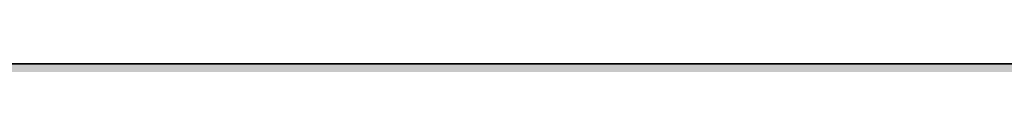
# Model space of a CAD drawing. Units: inches. Extents: x 2091 to 2899, y 967 to 2217.
# Tile 102 of 256: x 2252.951 to 2253.5204, y 1099.9191 to 1099.9191. Entities that reach past the tile are written whole.
import ezdxf

# ---------------------------------------------------------------- set-up
doc = ezdxf.new("R2010")
doc.units = ezdxf.units.IN
doc.layers.add('A-WALL-PATT', color=141, linetype='Continuous', lineweight=13, true_color=0xadddf7)
doc.layers.add('L-SITE-WALL', color=7, linetype='Continuous', lineweight=35)

msp = doc.modelspace()

# ---------------------------------------------------------------- hatches: boundary and pattern name
at = {"layer": 'A-WALL-PATT'}
h = msp.add_hatch(color=256, dxfattribs=at)
h.dxf.hatch_style = 1
h.paths.add_polyline_path([(2212.1436, 1941.41906), (2387.6436, 1941.41906), (2387.6436, 1824.41906), (2392.1436, 1824.41906), (2392.1436, 1941.41906), (2609.6436, 1941.41906), (2609.6436, 1825.91906), (2614.1436, 1825.91906), (2614.1436, 1941.41906), (2794.1436, 1941.41906), (2794.1436, 1928.76217), (2803.1436, 1928.76217), (2803.1436, 2050.91906), (2203.1436, 2050.91906), (2203.1436, 1900.75786), (2212.1436, 1900.75786)])
h.paths.add_polyline_path([(2212.1436, 1945.91906), (2212.1436, 2041.91906), (2794.1436, 2041.91906), (2794.1436, 1945.91906), (2402.24824, 1945.91906), (2401.10243, 1945.77583), (2398.70243, 1945.77583)], flags=16)
h.paths.add_polyline_path([(2230.22986, 1948.06279), (2227.34986, 1949.50279), (2225.90986, 1951.90279), (2223.98986, 1952.86279), (2223.02986, 1955.26279), (2222.06986, 1959.58279), (2222.06986, 1963.42279), (2223.02986, 1965.66279), (2223.98986, 1965.34279), (2225.58591, 1963.86075), (2226.91153, 1964.95726), (2226.94886, 1965.93879), (2227.77832, 1966.95214), (2228.19992, 1968.8787), (2230.70986, 1964.86279), (2233.58986, 1966.30279), (2233.60731, 1966.33187), (2233.77266, 1964.9382), (2234.6338, 1963.67647), (2235.02986, 1963.90279), (2236.28203, 1965.57236), (2235.98986, 1962.94279), (2237.95451, 1957.54), (2238.38986, 1957.90279), (2239.21586, 1960.30579), (2238.65457, 1966.38496), (2238.69279, 1966.43807), (2238.84058, 1967.49971), (2238.78029, 1967.68749), (2238.88054, 1967.78676), (2238.66686, 1966.25179), (2239.21586, 1960.30579), (2238.38986, 1957.90279), (2236.94986, 1956.70279), (2234.54986, 1949.98279)], flags=0)
h.paths.add_polyline_path([(2278.01197, 1948.06279), (2276.49643, 1947.87335), (2275.84983, 1947.68861), (2274.65197, 1947.10279)], flags=0)
h.paths.add_polyline_path([(2269.85197, 1955.74279), (2268.27618, 1956.62933), (2270.8673, 1956.3484), (2269.37197, 1958.14279), (2268.71496, 1959.19233), (2270.56983, 1958.72861), (2268.58073, 1961.90609), (2270.81197, 1960.89188), (2270.81197, 1963.42279), (2271.39331, 1964.77926), (2270.29176, 1966.1562), (2271.77197, 1965.66279), (2272.14139, 1966.52476), (2273.92983, 1965.92861), (2275.63039, 1968.0543), (2276.33194, 1966.72186), (2276.52043, 1966.95214), (2276.94203, 1968.8787), (2277.73429, 1967.61108), (2278.13989, 1969.46452), (2279.65912, 1967.03374), (2280.41197, 1966.78279), (2280.9493, 1967.58879), (2281.60983, 1967.36861), (2282.13327, 1968.15376), (2282.34924, 1966.33344), (2282.34985, 1966.33259), (2283.40755, 1968.09542), (2283.71263, 1965.52402), (2284.32022, 1964.63379), (2284.51181, 1964.88924), (2284.23497, 1965.70479), (2284.50047, 1967.31896), (2284.90794, 1965.41742), (2285.39631, 1966.06858), (2285.43283, 1966.29061), (2285.47334, 1966.17128), (2286.35392, 1967.34539), (2286.22201, 1966.15817), (2287.66349, 1968.08015), (2287.71397, 1968.44279), (2288.4816, 1969.01668), (2288.57399, 1968.7289), (2288.91746, 1969.06904), (2288.60683, 1966.83761), (2288.92873, 1963.35131), (2288.93497, 1963.35679), (2288.92973, 1963.34042), (2289.01528, 1962.41387), (2290.11122, 1963.87513), (2290.13283, 1963.94261), (2290.21767, 1964.01706), (2290.11122, 1963.87513), (2289.15583, 1960.89161), (2288.59404, 1959.25723), (2288.57197, 1959.10279), (2289.53197, 1960.54279), (2290.01197, 1962.46279), (2290.19184, 1962.64266), (2289.76983, 1959.68861), (2286.88983, 1957.28861), (2284.48983, 1950.56861), (2283.31466, 1950.04631), (2283.29197, 1949.98279), (2280.29006, 1948.64861), (2281.12983, 1948.64861), (2282.56983, 1948.16861), (2283.20473, 1948.06279), (2278.97197, 1948.06279), (2276.09197, 1949.50279), (2274.65197, 1951.90279), (2272.73197, 1952.86279)], flags=0)
h.paths.add_polyline_path([(2271.15887, 1958.02177), (2272.96983, 1955.84861), (2272.00983, 1960.16861), (2272.00983, 1964.00861), (2272.62443, 1965.44266), (2274.32802, 1963.86075), (2275.65365, 1964.95726), (2275.63774, 1964.53909), (2277.41223, 1966.00689), (2277.03297, 1965.15679), (2276.82992, 1964.9756), (2276.76601, 1963.29501), (2277.44964, 1962.66022), (2279.45197, 1964.86279), (2282.33197, 1966.30279), (2283.52983, 1966.88861), (2283.29451, 1966.77095), (2283.91299, 1963.8847), (2284.89925, 1964.44827), (2284.73197, 1962.94279), (2286.69662, 1957.54), (2287.13197, 1957.90279), (2287.54191, 1959.09539), (2287.7794, 1958.44231), (2285.68274, 1956.6951), (2285.8765, 1959.79534), (2284.73197, 1962.94279), (2284.89925, 1964.44827), (2283.91299, 1963.8847), (2284.22383, 1962.43412), (2283.42436, 1963.60548), (2281.60983, 1962.56861), (2281.12983, 1960.16861), (2282.08983, 1956.32861), (2283.04983, 1952.96861), (2282.56983, 1950.56861), (2280.16983, 1948.64861), (2279.88332, 1948.79187), (2278.97197, 1948.06279), (2278.97197, 1949.02279), (2278.67231, 1949.39737), (2277.28983, 1950.08861), (2275.84983, 1952.48861), (2273.92983, 1953.44861), (2272.48983, 1954.88861), (2271.92165, 1954.88861), (2271.77197, 1955.26279)], flags=0)
h.paths.add_polyline_path([(2311.99415, 1955.74279), (2312.06272, 1955.67422), (2312.0551, 1955.7085)], flags=0)
h.paths.add_polyline_path([(2331.95615, 1963.95179), (2333.39615, 1965.39179), (2331.07715, 1963.35679), (2330.9986, 1963.11152)], flags=0)
h.paths.add_polyline_path([(2310.55415, 1954.30279), (2307.03981, 1956.27994), (2310.7629, 1955.87628), (2312.47415, 1953.82279), (2313.43415, 1951.42279), (2315.35415, 1950.46279), (2316.79415, 1948.06279), (2317.46615, 1947.72679), (2319.36869, 1947.96461), (2317.75415, 1949.98279), (2317.56953, 1950.61048), (2316.79415, 1951.90279), (2314.87415, 1952.86279), (2313.91415, 1955.26279), (2311.51415, 1958.14279), (2309.37549, 1961.55917), (2311.51415, 1960.33708), (2311.51415, 1961.98279), (2310.60467, 1963.11963), (2311.72661, 1962.47853), (2312.41833, 1964.09256), (2312.25596, 1964.29552), (2313.19415, 1963.98279), (2313.91415, 1965.66279), (2314.64678, 1965.41858), (2315.35415, 1966.30279), (2316.79415, 1967.74279), (2316.15744, 1966.9469), (2317.03411, 1965.28186), (2317.2226, 1965.51214), (2317.77705, 1968.04577), (2318.47411, 1966.72186), (2318.6626, 1966.95214), (2319.0842, 1968.8787), (2321.20705, 1965.48215), (2322.16142, 1966.9137), (2322.55415, 1966.78279), (2322.78599, 1967.13056), (2322.88165, 1966.32429), (2323.31204, 1965.72174), (2323.65129, 1965.89136), (2324.3965, 1967.13338), (2324.65694, 1964.9382), (2324.97199, 1964.47661), (2325.38728, 1967.0015), (2325.94081, 1964.41835), (2327.22893, 1966.13584), (2327.16632, 1965.57236), (2328.05914, 1966.76278), (2328.22458, 1966.24749), (2329.66797, 1967.67691), (2329.66458, 1967.68749), (2329.76482, 1967.78676), (2329.55115, 1966.25179), (2330.10015, 1960.30579), (2329.33281, 1958.07347), (2329.31306, 1957.93523), (2329.63415, 1958.20279), (2330.23415, 1959.10279), (2330.71415, 1961.02279), (2331.03415, 1961.34279), (2330.71415, 1959.10279), (2329.63415, 1958.20279), (2329.27415, 1957.66279), (2327.71211, 1956.3611), (2325.43415, 1949.98279), (2324.33377, 1949.49374), (2323.99415, 1948.54279), (2319.67415, 1946.62279), (2316.79415, 1948.06279), (2315.35415, 1950.46279), (2313.43415, 1951.42279)], flags=0)
h.paths.add_polyline_path([(2321.33568, 1947.95202), (2321.11415, 1948.06279), (2321.11415, 1949.02279), (2319.19415, 1951.42279), (2316.79415, 1959.58279), (2316.66324, 1959.58279), (2315.35415, 1958.14279), (2314.39415, 1958.14279), (2313.1483, 1958.70908), (2312.95415, 1959.58279), (2312.95415, 1960.89188), (2315.83415, 1959.58279), (2316.66324, 1959.58279), (2317.31471, 1960.29941), (2315.0302, 1962.42075), (2316.35582, 1963.51726), (2316.37234, 1963.95162), (2316.4702, 1963.86075), (2317.79582, 1964.95726), (2317.75522, 1963.88969), (2319.17515, 1965.15679), (2319.49841, 1965.88137), (2321.11415, 1965.34279), (2323.23589, 1962.37236), (2325.68635, 1963.77262), (2325.54279, 1962.48058), (2325.19878, 1963.49401), (2324.47851, 1963.08243), (2324.92601, 1960.99412), (2324.07809, 1962.23647), (2322.41479, 1961.28602), (2322.07415, 1959.58279), (2323.03415, 1955.74279), (2323.99415, 1952.38279), (2323.51415, 1949.98279), (2322.14272, 1948.88565), (2322.07415, 1948.54279)], flags=0)
h.paths.add_polyline_path([(2320.20748, 1963.33746), (2320.15415, 1963.42279), (2320.39415, 1963.54279)], flags=0)
h.paths.add_polyline_path([(2353.85053, 1965.8105), (2354.03053, 1965.7505), (2354.33053, 1966.4505), (2354.33053, 1966.9305)], flags=0)
h.paths.add_polyline_path([(2359.02058, 1969.02641), (2359.09838, 1968.90193), (2359.23353, 1969.5195), (2359.23353, 1969.9995)], flags=0)
h.paths.add_polyline_path([(2358.25669, 1966.68167), (2357.9836, 1966.34803), (2358.21127, 1966.14617), (2358.41049, 1966.38957)], flags=0)
h.paths.add_polyline_path([(2357.76847, 1966.05878), (2357.7322, 1965.10497), (2357.75105, 1965.12056), (2357.76953, 1965.6065), (2357.76953, 1966.05784)], flags=0)
h.paths.add_polyline_path([(2359.11153, 1965.3045), (2359.11153, 1964.8245), (2359.84453, 1966.4675), (2359.84453, 1966.9475)], flags=0)
h.paths.add_polyline_path([(2360.22368, 1966.62145), (2360.69853, 1969.3625), (2360.69853, 1969.8425), (2360.21053, 1967.0255), (2360.21053, 1966.6425)], flags=0)
h.paths.add_polyline_path([(2363.45053, 1967.8905), (2363.45053, 1968.3705), (2362.49053, 1966.9305), (2362.65604, 1966.69878)], flags=0)
h.paths.add_polyline_path([(2364.47552, 1966.07883), (2365.85053, 1968.3705), (2365.85053, 1968.8505), (2364.42798, 1966.47958)], flags=0)
h.paths.add_polyline_path([(2366.31353, 1965.8525), (2366.36671, 1965.69583), (2366.80253, 1968.3455), (2366.80253, 1968.8255)], flags=0)
h.paths.add_polyline_path([(2367.16531, 1965.80354), (2367.29053, 1966.9305), (2367.29053, 1967.4105), (2367.1027, 1965.72007)], flags=0)
h.paths.add_polyline_path([(2370.03653, 1959.9735), (2371.01353, 1963.0245), (2371.01353, 1963.5045), (2370.03653, 1960.4535)], flags=0)
h.paths.add_polyline_path([(2371.61053, 1960.2105), (2372.57053, 1961.6505), (2372.57053, 1962.1305), (2371.80253, 1960.9785)], flags=0)
h.paths.add_polyline_path([(2350.87367, 1956.00509), (2351.93053, 1955.8905), (2354.49053, 1953.3305), (2353.85053, 1954.9305), (2351.45053, 1957.8105), (2347.93553, 1963.4255), (2347.93553, 1963.9055), (2351.45053, 1958.2905), (2353.70507, 1955.58505), (2352.89053, 1959.2505), (2352.89053, 1959.7305), (2352.89053, 1961.92479), (2356.73053, 1959.7305), (2358.45447, 1961.62684), (2354.81053, 1965.0105), (2355.03086, 1965.28591), (2358.69109, 1961.88712), (2361.53053, 1965.0105), (2364.3765, 1966.43348), (2364.52439, 1965.18691), (2365.45447, 1963.82418), (2365.88107, 1964.06795), (2365.37053, 1966.4505), (2365.37053, 1966.9305), (2366.81053, 1960.2105), (2366.81053, 1959.7305), (2366.38871, 1952.98141), (2367.77053, 1956.8505), (2368.64123, 1957.57608), (2366.81053, 1962.6105), (2366.81053, 1963.0905), (2368.77518, 1957.68771), (2369.21053, 1958.0505), (2370.00159, 1960.35187), (2369.47523, 1966.05267), (2369.51346, 1966.10578), (2369.51417, 1966.11091), (2369.47523, 1966.53267), (2369.51346, 1966.58578), (2369.61463, 1967.31259), (2369.18253, 1968.6585), (2369.18253, 1969.1385), (2369.60096, 1967.83519), (2369.7012, 1967.93447), (2369.71795, 1968.05474), (2370.14518, 1968.37414), (2369.77871, 1968.01122), (2369.7012, 1967.45447), (2370.46816, 1968.214), (2369.67494, 1967.26577), (2369.51417, 1966.11091), (2370.03653, 1960.4535), (2370.03653, 1959.9735), (2369.44176, 1958.24319), (2370.65053, 1959.2505), (2371.04582, 1962.01756), (2371.13053, 1962.1305), (2370.65053, 1958.7705), (2367.77053, 1956.3705), (2365.37053, 1949.6505), (2362.0791, 1948.18764), (2363.45053, 1947.7305), (2361.05053, 1947.7305), (2360.09053, 1947.7305), (2357.10386, 1947.35717), (2360.09053, 1948.2105), (2358.17053, 1949.1705), (2356.73053, 1951.5705), (2354.81053, 1952.5305), (2351.93053, 1955.4105)], flags=0)
h.paths.add_polyline_path([(2361.05053, 1948.6905), (2359.13053, 1951.0905), (2356.73053, 1959.2505), (2355.77053, 1959.2505), (2352.89053, 1960.55959), (2352.89053, 1961.44479), (2355.89053, 1959.7305), (2356.73053, 1959.7305), (2356.83719, 1959.36783), (2361.53053, 1964.5305), (2363.24842, 1965.38945), (2364.92531, 1963.0418), (2362.49053, 1961.6505), (2362.06386, 1959.51717), (2362.97053, 1955.8905), (2363.93053, 1952.5305), (2363.93053, 1952.0505), (2363.45053, 1949.6505), (2361.05053, 1947.7305)], flags=0)
h.paths.add_polyline_path([(2359.13053, 1951.5705), (2359.29053, 1951.3705), (2361.05053, 1954.4505), (2361.05053, 1954.9305)], flags=0)
h.paths.add_polyline_path([(2357.21953, 1966.5455), (2356.79253, 1968.8145), (2356.79253, 1969.2945), (2357.21953, 1967.0255)], flags=0)
h.paths.add_polyline_path([(2361.05053, 1954.4505), (2361.53053, 1958.7705), (2361.53053, 1959.2505), (2361.05053, 1954.9305)], flags=0)
h.paths.add_polyline_path([(2402.54829, 1948.48608), (2402.30243, 1948.41583), (2402.59043, 1948.41583)], flags=0)
h.paths.add_polyline_path([(2394.14243, 1956.09583), (2395.68505, 1954.55321), (2396.7205, 1953.97068), (2396.06243, 1955.61583), (2395.24138, 1956.6011), (2395.8789, 1956.44171), (2395.10243, 1959.93583), (2395.10243, 1963.77583), (2396.06243, 1966.01583), (2397.02243, 1965.69583), (2398.61848, 1964.21379), (2399.94411, 1965.3103), (2399.98143, 1966.29183), (2400.81089, 1967.30518), (2401.23249, 1969.23174), (2403.53795, 1965.54301), (2403.94198, 1967.38932), (2404.70243, 1967.13583), (2405.46033, 1966.07478), (2406.62243, 1966.65583), (2406.63988, 1966.68491), (2406.80523, 1965.29124), (2406.92569, 1965.11475), (2407.34243, 1964.97583), (2407.87433, 1965.77367), (2408.1691, 1964.39805), (2409.31461, 1965.9254), (2409.21746, 1965.05105), (2409.44523, 1963.13124), (2410.30637, 1961.86951), (2410.70243, 1962.09583), (2411.44227, 1963.08228), (2411.16543, 1963.89783), (2411.61643, 1966.63976), (2411.72536, 1966.79111), (2411.87315, 1967.85275), (2411.81286, 1968.04053), (2411.91311, 1968.1398), (2411.69943, 1966.60483), (2412.24843, 1960.65883), (2413.22543, 1963.70983), (2414.3779, 1964.72116), (2414.51315, 1965.69275), (2414.45286, 1965.88053), (2414.55311, 1965.9798), (2414.3779, 1964.72116), (2414.51982, 1964.8457), (2414.36536, 1964.63111), (2414.33943, 1964.44483), (2414.88843, 1958.49883), (2414.06243, 1956.09583), (2412.62243, 1954.89583), (2410.17137, 1948.03285), (2410.01672, 1948.0844), (2405.90243, 1946.25583), (2405.90243, 1947.21583), (2405.20425, 1948.08856), (2404.22243, 1948.41583), (2403.26243, 1948.41583), (2400.38243, 1949.85583), (2399.66243, 1951.05583), (2397.98243, 1952.73583), (2397.02243, 1953.21583), (2395.68505, 1954.55321), (2392.65678, 1956.25691)], flags=0)
h.paths.add_polyline_path([(2409.08565, 1964.40744), (2409.13036, 1964.27572), (2409.26243, 1964.49583)], flags=0)
h.paths.add_polyline_path([(2397.74243, 1961.61583), (2398.70243, 1963.85583), (2399.66243, 1963.53583), (2401.42656, 1965.74099), (2401.79142, 1966.5588), (2402.07143, 1965.07083), (2402.83551, 1964.39337), (2403.2624, 1964.9149), (2403.33812, 1964.77109), (2402.61552, 1963.97622), (2402.49861, 1960.90224), (2403.543, 1959.93245), (2404.4132, 1960.88968), (2404.70243, 1962.33583), (2407.91635, 1964.17235), (2409.52021, 1961.92694), (2410.98708, 1957.89304), (2411.42243, 1958.25583), (2412.04796, 1960.07562), (2412.41034, 1959.07909), (2411.67562, 1958.46682), (2411.66243, 1958.25583), (2411.62607, 1958.42553), (2409.98243, 1957.05583), (2407.58243, 1950.33583), (2403.26243, 1948.41583), (2403.26243, 1949.37583), (2401.34243, 1951.77583), (2399.41651, 1958.32398), (2397.74243, 1959.08492), (2397.74243, 1959.97012), (2397.10243, 1960.33583), (2397.74243, 1960.04492)], flags=0)
h.paths.add_polyline_path([(2405.90243, 1952.97583), (2405.95043, 1953.40783), (2406.01672, 1953.17583)], flags=0)
h.paths.add_polyline_path([(2449.81778, 1967.11401), (2449.75232, 1967.13583), (2449.7937, 1967.0779)], flags=0)
h.paths.add_polyline_path([(2451.6977, 1966.61812), (2451.74089, 1966.69012), (2451.69205, 1966.6657)], flags=0)
h.paths.add_polyline_path([(2454.34363, 1965.73757), (2455.75232, 1967.61583), (2455.99232, 1968.09583), (2454.3645, 1965.9254)], flags=0)
h.paths.add_polyline_path([(2457.54732, 1968.86383), (2457.78732, 1969.34383), (2457.05432, 1968.79583), (2457.00762, 1968.46034)], flags=0)
h.paths.add_polyline_path([(2456.92178, 1967.85666), (2456.80224, 1968.22902), (2456.723, 1967.6598)], flags=0)
h.paths.add_polyline_path([(2457.30232, 1967.37683), (2457.54232, 1967.85683), (2456.81032, 1966.83983), (2456.74052, 1966.70022), (2456.74902, 1966.60811)], flags=0)
h.paths.add_polyline_path([(2458.27532, 1963.70983), (2458.15534, 1963.33515), (2460.35432, 1965.26483), (2460.59432, 1965.74483)], flags=0)
h.paths.add_polyline_path([(2458.39232, 1962.81583), (2458.36409, 1962.61819), (2459.59232, 1964.25583), (2459.83232, 1964.73583)], flags=0)
h.paths.add_polyline_path([(2459.35232, 1962.81583), (2459.27232, 1962.49583), (2460.07232, 1963.29583), (2460.31232, 1963.77583)], flags=0)
h.paths.add_polyline_path([(2458.68032, 1960.60783), (2458.63232, 1960.41583), (2459.59232, 1961.85583), (2459.83232, 1962.33583)], flags=0)
h.paths.add_polyline_path([(2437.83817, 1956.24265), (2439.19232, 1956.09583), (2441.35232, 1953.93583), (2440.87232, 1955.13583), (2438.47232, 1958.01583), (2438.07156, 1958.65602), (2438.71232, 1958.49583), (2440.6396, 1956.18311), (2439.91232, 1959.45583), (2439.91232, 1963.29583), (2441.35232, 1966.65583), (2441.59232, 1967.13583), (2441.11232, 1966.01583), (2442.07232, 1965.69583), (2443.98899, 1968.09167), (2444.24132, 1966.75083), (2444.9168, 1966.15192), (2445.67657, 1967.08014), (2446.25532, 1969.72483), (2446.49532, 1970.20483), (2446.28238, 1969.23174), (2447.36267, 1967.50327), (2447.72032, 1969.56783), (2447.96032, 1970.04783), (2447.48548, 1967.30678), (2448.79232, 1965.21583), (2448.47232, 1964.86383), (2448.55232, 1964.73583), (2451.45205, 1966.1857), (2451.61512, 1964.81124), (2452.30792, 1963.79617), (2453.23451, 1964.32565), (2454.07232, 1960.41583), (2453.62869, 1953.31765), (2454.79232, 1956.57583), (2455.03232, 1957.05583), (2455.71884, 1957.62793), (2453.83232, 1962.81583), (2453.94097, 1963.79362), (2453.33532, 1965.57783), (2453.82432, 1968.55083), (2454.06432, 1969.03083), (2453.57532, 1966.05783), (2454.04033, 1964.68792), (2453.83232, 1962.81583), (2455.71884, 1957.62793), (2456.36721, 1958.16824), (2457.05832, 1960.17883), (2457.29832, 1960.65883), (2456.47232, 1958.25583), (2457.71773, 1959.29367), (2457.67232, 1958.97583), (2454.88995, 1956.65719), (2453.61414, 1953.08492), (2453.59232, 1952.73583), (2453.35232, 1952.25583), (2453.3596, 1952.3722), (2452.63232, 1950.33583), (2452.39232, 1949.85583), (2449.20375, 1948.43869), (2450.71232, 1947.93583), (2448.07232, 1947.93583), (2447.11232, 1947.93583), (2444.55232, 1947.61583), (2447.1996, 1948.3722), (2445.19232, 1949.37583), (2443.75232, 1951.77583), (2441.83232, 1952.73583), (2438.95232, 1955.61583)], flags=0)
h.paths.add_polyline_path([(2443.99232, 1959.93583), (2444.04032, 1959.77263), (2444.12155, 1959.86199)], flags=0)
h.paths.add_polyline_path([(2442.91232, 1959.93583), (2443.03232, 1959.93583), (2442.44566, 1960.2025)], flags=0)
h.paths.add_polyline_path([(2444.98294, 1965.01968), (2445.27932, 1965.26483), (2445.51932, 1965.74483), (2444.994, 1965.3103)], flags=0)
h.paths.add_polyline_path([(2446.13332, 1965.02983), (2446.33037, 1965.4715), (2444.97032, 1964.25783), (2444.73032, 1963.77783)], flags=0)
h.paths.add_polyline_path([(2442.79232, 1959.45583), (2443.75232, 1959.45583), (2446.15232, 1951.29583), (2446.41232, 1951.75083), (2446.39232, 1951.77583), (2448.0806, 1954.73032), (2448.55232, 1958.97583), (2441.83232, 1965.21583), (2442.15495, 1965.61911), (2448.79232, 1959.45583), (2448.31232, 1955.13583), (2448.07232, 1954.65583), (2446.41232, 1951.75083), (2448.31232, 1949.37583), (2448.31232, 1948.41583), (2450.54089, 1950.19869), (2450.95232, 1952.25583), (2449.99232, 1955.61583), (2449.03232, 1959.45583), (2449.51232, 1961.85583), (2449.75232, 1962.33583), (2449.6749, 1961.94874), (2452.99451, 1963.84565), (2453.06441, 1963.51941), (2452.88461, 1963.78285), (2449.6749, 1961.94874), (2449.27232, 1959.93583), (2450.23232, 1956.09583), (2451.19232, 1952.73583), (2450.71232, 1950.33583), (2450.47232, 1949.85583), (2448.07232, 1947.93583), (2448.07232, 1948.53583), (2445.43232, 1949.85583), (2443.99232, 1952.25583), (2442.07232, 1953.21583), (2441.11232, 1955.61583), (2440.15232, 1959.93583), (2440.15232, 1960.65583)], flags=0)
h.paths.add_polyline_path([(2456.69232, 1966.98583), (2457.60832, 1968.08083), (2457.84832, 1968.56083), (2456.93232, 1967.46583)], flags=0)
h.paths.add_polyline_path([(2489.89657, 1966.58024), (2489.94295, 1966.18935), (2490.74749, 1967.53025), (2491.31912, 1968.95116)], flags=0)
h.paths.add_polyline_path([(2473.56247, 1956.40713), (2477.13998, 1956.01926), (2476.95533, 1956.24083), (2475.10805, 1957.28011), (2476.34749, 1956.97025), (2475.1869, 1958.82422), (2476.91912, 1958.39116), (2475.41164, 1960.79927), (2477.78749, 1959.71934), (2477.78749, 1962.25025), (2477.6374, 1962.43786), (2477.82255, 1962.33206), (2478.35912, 1963.58406), (2478.35912, 1963.67116), (2477.32435, 1964.96463), (2478.71483, 1964.50114), (2479.31912, 1965.91116), (2480.27912, 1965.59116), (2481.78397, 1967.47221), (2482.11649, 1965.70525), (2482.88056, 1965.02778), (2483.20931, 1965.42941), (2483.22017, 1965.71509), (2483.07594, 1965.98902), (2483.71176, 1966.76581), (2484.13049, 1968.67925), (2484.70212, 1970.10016), (2484.48918, 1969.12707), (2486.5029, 1965.90511), (2487.38749, 1965.61025), (2488.15342, 1966.75914), (2488.71702, 1965.97011), (2489.20009, 1966.21164), (2489.33067, 1965.11099), (2490.3939, 1963.62246), (2490.66077, 1963.77496), (2490.49391, 1964.55364), (2490.92306, 1963.92484), (2491.31912, 1964.15116), (2491.33339, 1964.17018), (2491.21049, 1964.53225), (2491.28176, 1964.96554), (2491.42579, 1964.29338), (2494.07648, 1967.82763), (2494.49792, 1966.51494), (2494.59817, 1966.61422), (2494.68949, 1967.27025), (2495.10675, 1967.5822), (2495.12984, 1967.74807), (2495.06955, 1967.93585), (2495.1698, 1968.03513), (2495.03178, 1967.04363), (2495.75382, 1967.75868), (2494.98205, 1966.68644), (2494.95612, 1966.50016), (2495.47902, 1960.83685), (2495.91049, 1962.18425), (2496.48212, 1963.60516), (2496.07269, 1962.32659), (2496.7689, 1962.93754), (2496.59912, 1962.71116), (2496.11912, 1959.35116), (2496.73287, 1960.27179), (2496.98749, 1961.29025), (2497.55912, 1962.71116), (2497.07912, 1960.79116), (2496.50749, 1959.37025), (2495.54749, 1957.93025), (2492.75884, 1955.60638), (2490.83912, 1950.23116), (2490.26749, 1948.81025), (2485.94749, 1946.89025), (2483.06749, 1948.33025), (2481.62749, 1950.73025), (2479.70749, 1951.69025), (2476.82749, 1954.57025)], flags=0)
h.paths.add_polyline_path([(2485.57697, 1948.31339), (2485.55912, 1948.31116), (2485.57876, 1948.31116)], flags=0)
h.paths.add_polyline_path([(2478.64506, 1954.55116), (2478.10904, 1956.96326), (2479.31912, 1955.51116), (2480.27912, 1953.11116), (2482.19912, 1952.15116), (2483.63912, 1949.75116), (2486.51912, 1948.31116), (2486.51912, 1949.27116), (2484.73931, 1951.49593), (2484.02749, 1950.25025), (2481.62749, 1958.41025), (2482.37515, 1959.23267), (2482.19912, 1959.83116), (2483.19757, 1960.92946), (2479.70749, 1964.17025), (2480.60336, 1965.29008), (2481.87517, 1964.10911), (2482.66639, 1964.76358), (2482.61536, 1963.4218), (2482.9892, 1963.07466), (2484.00849, 1963.98425), (2484.68361, 1965.49751), (2484.58012, 1965.40516), (2485.35727, 1967.14711), (2485.12065, 1965.7812), (2486.42749, 1963.69025), (2488.14538, 1964.5492), (2489.82227, 1962.20155), (2490.74749, 1962.73025), (2491.99966, 1964.39981), (2492.07605, 1965.08726), (2492.21289, 1964.68412), (2492.48537, 1965.04743), (2492.27912, 1963.19116), (2494.24377, 1957.78837), (2494.5625, 1958.05398), (2494.93349, 1959.13325), (2495.50512, 1960.55416), (2494.67912, 1958.15116), (2494.10749, 1956.73025), (2494.5625, 1958.05398), (2493.40854, 1957.09235), (2491.70749, 1961.77025), (2491.99966, 1964.39981), (2490.74749, 1962.73025), (2487.71203, 1960.9957), (2487.47912, 1959.83116), (2488.43912, 1955.99116), (2489.39912, 1952.63116), (2488.91912, 1950.23116), (2488.57692, 1949.9574), (2488.34749, 1948.81025), (2487.65172, 1948.25363), (2487.47912, 1948.31116), (2486.51912, 1948.31116), (2483.63912, 1949.75116), (2482.19912, 1952.15116), (2480.27912, 1953.11116), (2478.83912, 1954.55116)], flags=0)
h.paths.add_polyline_path([(2526.64825, 1966.98752), (2526.51734, 1967.03116), (2526.6001, 1966.9153)], flags=0)
h.paths.add_polyline_path([(2528.47064, 1966.44666), (2528.57449, 1966.61973), (2528.45707, 1966.56102)], flags=0)
h.paths.add_polyline_path([(2534.13334, 1967.49616), (2534.15669, 1967.54285), (2534.05984, 1967.4083)], flags=0)
h.paths.add_polyline_path([(2536.16192, 1964.0506), (2535.15734, 1962.71116), (2535.10087, 1962.31587), (2536.11734, 1963.67116), (2536.42053, 1964.27754)], flags=0)
h.paths.add_polyline_path([(2535.15734, 1959.83116), (2536.11734, 1961.27116), (2536.59734, 1962.23116), (2535.25334, 1960.21516)], flags=0)
h.paths.add_polyline_path([(2513.24904, 1956.2848), (2516.22118, 1955.96256), (2514.99734, 1957.43116), (2514.19582, 1958.71154), (2515.47734, 1958.39116), (2516.93189, 1956.64571), (2516.43734, 1958.87116), (2516.43734, 1962.71116), (2516.87269, 1963.72697), (2515.34643, 1965.6348), (2517.39734, 1964.95116), (2517.87734, 1966.07116), (2518.35734, 1967.03116), (2517.87734, 1965.91116), (2518.83734, 1965.59116), (2520.48659, 1967.65272), (2520.76634, 1966.16616), (2521.53042, 1965.48869), (2521.78144, 1965.79537), (2521.80091, 1966.30727), (2521.4778, 1966.92094), (2521.24634, 1967.12616), (2521.1777, 1967.49091), (2521.4778, 1966.92094), (2522.01042, 1966.44869), (2522.25739, 1966.75042), (2522.78034, 1969.14016), (2523.26034, 1970.10016), (2523.0474, 1969.12707), (2524.67313, 1966.5259), (2526.03734, 1966.07116), (2526.79524, 1965.01011), (2527.97707, 1965.60102), (2528.14014, 1964.22657), (2528.66459, 1963.45816), (2529.38862, 1963.87189), (2529.32967, 1964.14699), (2529.48128, 1963.92484), (2529.87734, 1964.15116), (2529.98401, 1964.29338), (2529.78905, 1965.20318), (2530.0624, 1964.3979), (2532.80248, 1968.05135), (2533.14777, 1966.97585), (2533.24802, 1967.07513), (2533.33934, 1967.73116), (2533.67285, 1967.98049), (2533.72802, 1968.03513), (2533.51434, 1966.50016), (2534.02472, 1960.9725), (2534.56034, 1962.64516), (2535.04034, 1963.60516), (2534.06334, 1960.55416), (2533.23734, 1958.15116), (2534.28815, 1959.02684), (2534.19734, 1958.39116), (2531.5126, 1956.15387), (2529.39734, 1950.23116), (2528.91734, 1949.27116), (2526.44877, 1948.17402), (2527.47734, 1947.83116), (2530.35734, 1947.35116), (2524.59734, 1947.35116), (2521.71734, 1948.79116), (2520.27734, 1951.19116), (2518.35734, 1952.15116), (2515.47734, 1955.03116)], flags=0)
h.paths.add_polyline_path([(2523.93476, 1967.19031), (2523.61951, 1966.48369), (2523.7705, 1966.24211)], flags=0)
h.paths.add_polyline_path([(2518.83734, 1953.11116), (2517.87734, 1955.51116), (2516.88498, 1959.97678), (2516.91734, 1959.96207), (2516.91734, 1962.02545), (2520.75734, 1959.83116), (2522.02495, 1961.22553), (2518.35734, 1964.63116), (2519.00259, 1965.43772), (2520.43339, 1964.10911), (2521.30112, 1964.82687), (2521.24516, 1963.35533), (2525.63831, 1959.27598), (2526.03734, 1961.27116), (2529.39734, 1963.19116), (2530.64952, 1964.86073), (2530.66472, 1964.99755), (2530.69196, 1964.91731), (2531.08778, 1965.44507), (2530.94599, 1964.16894), (2530.69196, 1964.91731), (2529.39734, 1963.19116), (2526.3625, 1961.45697), (2526.03734, 1959.83116), (2526.99734, 1955.99116), (2527.95734, 1952.63116), (2527.47734, 1950.23116), (2527.13449, 1949.95687), (2526.97393, 1949.15409), (2526.69734, 1949.03116), (2524.59734, 1947.35116), (2524.59734, 1948.31116), (2524.27734, 1948.71116), (2522.19734, 1949.75116), (2520.75734, 1952.15116)], flags=0)
h.paths.add_polyline_path([(2520.27734, 1958.87116), (2520.85334, 1959.50476), (2523.15734, 1951.67116), (2524.61389, 1954.22013), (2524.59734, 1954.07116), (2522.67734, 1950.71116)], flags=0)
h.paths.add_polyline_path([(2559.37091, 1966.31116), (2559.39841, 1966.32491), (2559.40194, 1966.3453)], flags=0)
h.paths.add_polyline_path([(2549.77091, 1957.19116), (2552.65091, 1954.31116), (2552.13399, 1955.60347), (2550.61091, 1957.43116), (2547.09591, 1963.04616), (2545.77591, 1965.20616), (2549.29091, 1959.59116), (2551.69091, 1956.71116), (2550.79293, 1960.75206), (2550.73091, 1960.78025), (2550.73091, 1964.87116), (2551.69091, 1967.11116), (2552.65091, 1966.79116), (2554.24696, 1965.30911), (2555.03425, 1965.96034), (2555.58167, 1966.64461), (2555.60991, 1967.38716), (2556.43937, 1968.40051), (2556.86097, 1970.32707), (2559.37091, 1966.31116), (2560.69091, 1964.15116), (2562.40881, 1965.01011), (2561.65091, 1966.07116), (2560.33091, 1968.23116), (2561.7585, 1966.23254), (2562.34721, 1967.11561), (2562.43371, 1966.38657), (2563.1278, 1965.3696), (2563.57091, 1965.59116), (2563.58836, 1965.62024), (2563.36254, 1967.52354), (2563.72249, 1965.84379), (2565.06, 1968.07298), (2564.73286, 1965.12872), (2565.11758, 1963.33338), (2567.44462, 1966.43611), (2567.31561, 1967.83333), (2567.35384, 1967.88644), (2567.50163, 1968.94807), (2567.44134, 1969.13585), (2567.54159, 1969.23513), (2567.32791, 1967.70016), (2567.87691, 1961.75416), (2568.74669, 1964.47033), (2568.63561, 1965.67333), (2568.67384, 1965.72644), (2568.82163, 1966.78807), (2568.76134, 1966.97585), (2568.86159, 1967.07513), (2568.64791, 1965.54016), (2568.72613, 1964.69303), (2568.85391, 1964.80516), (2568.74669, 1964.47033), (2568.81724, 1963.70626), (2568.97091, 1963.91116), (2568.86607, 1963.17731), (2569.19691, 1959.59416), (2568.37091, 1957.19116), (2566.93091, 1955.99116), (2564.62027, 1949.52137), (2564.65091, 1949.51116), (2564.61662, 1949.51116), (2564.53091, 1949.27116), (2560.21091, 1947.35116), (2557.33091, 1948.79116), (2556.0452, 1950.93402), (2556.01091, 1950.95116), (2555.85662, 1951.2083), (2553.97091, 1952.15116), (2551.09091, 1955.03116), (2546.65014, 1957.52951)], flags=0)
h.paths.add_polyline_path([(2567.02579, 1959.33023), (2567.03501, 1959.30489), (2567.05091, 1959.35116)], flags=0)
h.paths.add_polyline_path([(2551.96829, 1962.51837), (2553.01091, 1964.95116), (2553.97091, 1964.63116), (2555.56696, 1963.14911), (2556.89258, 1964.24563), (2556.92991, 1965.22716), (2557.14398, 1965.48869), (2556.42007, 1966.13056), (2556.39142, 1966.10499), (2556.37991, 1966.16616), (2556.42007, 1966.13056), (2556.95191, 1966.60516), (2557.09214, 1966.91948), (2557.57087, 1966.01023), (2557.75937, 1966.24051), (2557.41791, 1964.68016), (2556.89258, 1964.24563), (2556.80709, 1961.99757), (2560.69091, 1958.39116), (2560.63553, 1957.8927), (2560.81091, 1957.19116), (2561.77091, 1953.83116), (2561.29091, 1951.43116), (2559.11042, 1949.68677), (2559.15648, 1949.62919), (2563.02652, 1951.34921), (2562.61091, 1949.27116), (2560.21091, 1947.35116), (2560.21091, 1948.31116), (2559.25091, 1949.51116), (2558.89091, 1949.51116), (2558.89091, 1949.96116), (2558.29091, 1950.71116), (2558.0537, 1951.51767), (2556.97091, 1952.87116), (2555.06788, 1959.34146), (2552.05091, 1961.06545), (2552.05091, 1962.47116)], flags=0)
h.paths.add_polyline_path([(2588.33005, 1958.39116), (2588.61025, 1958.11096), (2588.55336, 1958.36695)], flags=0)
h.paths.add_polyline_path([(2594.74545, 1950.49309), (2593.95753, 1953.17202), (2593.13005, 1954.55116), (2591.21005, 1955.51116), (2590.25005, 1957.91116), (2588.30903, 1960.24038), (2586.17731, 1961.20935), (2587.85005, 1960.79116), (2587.25342, 1961.74425), (2588.44131, 1961.06545), (2588.44131, 1962.65553), (2588.42168, 1962.66535), (2588.44131, 1962.71116), (2586.91404, 1964.62026), (2588.87709, 1963.72796), (2589.29005, 1964.69154), (2589.29005, 1966.07116), (2590.25005, 1968.31116), (2591.21005, 1967.99116), (2592.8061, 1966.50911), (2594.13172, 1967.60563), (2594.16905, 1968.58716), (2594.99851, 1969.60051), (2595.4201, 1971.52707), (2597.93005, 1967.51116), (2600.81005, 1968.95116), (2600.8275, 1968.98024), (2600.99285, 1967.58657), (2601.85399, 1966.32484), (2602.10714, 1966.4695), (2602.23635, 1967.25507), (2602.35672, 1966.69338), (2603.50222, 1968.22073), (2603.21005, 1965.59116), (2605.1747, 1960.18837), (2605.50689, 1960.4652), (2605.02602, 1965.67333), (2605.06425, 1965.72644), (2605.21203, 1966.78807), (2605.15174, 1966.97585), (2605.25199, 1967.07513), (2605.34331, 1967.73116), (2605.9529, 1968.1869), (2605.87475, 1969.03333), (2605.91298, 1969.08644), (2606.06077, 1970.14807), (2606.00048, 1970.33585), (2606.10073, 1970.43513), (2605.88705, 1968.90016), (2606.43605, 1962.95416), (2605.61005, 1960.55116), (2605.99704, 1960.87365), (2606.56431, 1962.64516), (2608.24149, 1964.11694), (2608.01005, 1963.19116), (2607.05005, 1961.75116), (2606.63149, 1961.40236), (2606.20131, 1958.39116), (2603.32131, 1955.99116), (2600.92131, 1949.27116), (2596.60131, 1947.35116), (2593.72131, 1948.79116), (2592.85731, 1950.23116), (2592.65005, 1950.23116)], flags=0)
h.paths.add_polyline_path([(2596.60131, 1947.35116), (2596.60131, 1948.31116), (2594.68131, 1950.71116), (2596.15495, 1953.29003), (2595.53005, 1954.07116), (2593.19923, 1961.99596), (2592.65134, 1962.50471), (2591.78015, 1963.00253), (2593.28299, 1964.24563), (2593.32031, 1965.22716), (2594.14977, 1966.24051), (2594.57137, 1968.16707), (2596.18265, 1965.58902), (2596.95127, 1966.43451), (2598.04131, 1966.07116), (2598.79921, 1965.01011), (2599.96131, 1965.59116), (2599.97876, 1965.62024), (2600.14411, 1964.22657), (2601.00526, 1962.96484), (2601.40131, 1963.19116), (2602.65349, 1964.86073), (2602.36131, 1962.23116), (2603.79275, 1958.29472), (2601.97764, 1953.21243), (2601.94621, 1952.70945), (2599.46876, 1951.60836), (2599.00131, 1949.27116)], flags=0)
h.paths.add_polyline_path([(2597.56131, 1958.87116), (2597.67097, 1959.41942), (2597.59505, 1958.7362)], flags=0)
h.paths.add_polyline_path([(2623.6663, 1961.25438), (2625.51916, 1960.79116), (2624.96554, 1961.67553), (2627.19916, 1960.66025), (2627.19916, 1961.15116), (2626.95916, 1962.23116), (2626.95916, 1963.49116), (2625.58232, 1965.21221), (2626.95916, 1964.42545), (2626.95916, 1965.83116), (2626.86916, 1965.86116), (2627.91916, 1968.31116), (2628.87916, 1967.99116), (2630.47521, 1966.50911), (2631.80084, 1967.60563), (2631.83816, 1968.58716), (2632.66762, 1969.60051), (2633.08922, 1971.52707), (2635.59916, 1967.51116), (2638.47916, 1968.95116), (2638.49661, 1968.98024), (2638.66196, 1967.58657), (2639.17627, 1966.83301), (2639.78022, 1967.83958), (2640.02583, 1966.69338), (2641.17134, 1968.22073), (2640.87916, 1965.59116), (2641.11426, 1964.94463), (2641.41134, 1965.34073), (2641.3081, 1964.41159), (2642.84381, 1960.18837), (2643.27916, 1960.55116), (2644.08474, 1962.89474), (2643.78387, 1966.15333), (2643.80683, 1966.18524), (2643.60068, 1968.41805), (2643.52281, 1968.66058), (2643.72988, 1970.14807), (2643.66959, 1970.33585), (2643.76984, 1970.43513), (2643.55616, 1968.90016), (2643.60068, 1968.41805), (2643.90959, 1967.45585), (2644.00984, 1967.55513), (2643.81174, 1966.13208), (2644.10516, 1962.95416), (2644.23877, 1961.35084), (2644.71916, 1961.75116), (2645.03285, 1962.2217), (2645.32216, 1963.12516), (2646.07642, 1963.78705), (2645.03285, 1962.2217), (2644.34516, 1960.07416), (2643.51916, 1957.67116), (2642.07916, 1956.47116), (2639.71961, 1949.86442), (2639.87553, 1949.83843), (2635.35916, 1947.83116), (2632.47916, 1949.27116), (2631.03916, 1951.67116), (2629.11916, 1952.63116), (2628.15916, 1955.03116), (2625.75916, 1957.91116)], flags=0)
h.paths.add_polyline_path([(2627.81631, 1956.57402), (2627.37371, 1958.56571), (2626.37631, 1959.76259), (2627.19916, 1959.35116), (2627.37371, 1958.56571), (2627.91916, 1957.91116), (2628.87916, 1955.51116), (2630.79916, 1954.55116), (2632.23916, 1952.15116), (2633.31502, 1951.61323), (2631.03916, 1959.35116), (2631.49783, 1959.85569), (2630.79916, 1962.23116), (2631.44987, 1962.94694), (2630.71521, 1963.62911), (2632.04084, 1964.72563), (2632.07816, 1965.70716), (2632.29224, 1965.96869), (2631.70534, 1966.48907), (2633.13644, 1967.76614), (2633.32922, 1968.64707), (2634.67472, 1966.49427), (2635.20847, 1967.08139), (2636.79916, 1966.55116), (2637.6764, 1967.86702), (2638.99395, 1966.02246), (2639.70534, 1966.42898), (2641.11916, 1959.83116), (2640.93007, 1956.80571), (2639.43916, 1952.63116), (2638.22746, 1952.09262), (2637.75916, 1949.75116), (2635.35916, 1947.83116), (2635.35916, 1948.79116), (2633.43916, 1951.19116), (2633.31502, 1951.61323), (2632.23916, 1952.15116), (2630.79916, 1954.55116), (2628.87916, 1955.51116)], flags=0)
h.paths.add_polyline_path([(2637.75916, 1953.83116), (2637.27916, 1955.51116), (2636.31916, 1959.35116), (2636.79916, 1961.75116), (2639.23395, 1963.14246), (2637.55706, 1965.49011), (2638.73889, 1966.08102), (2638.90196, 1964.70657), (2639.7631, 1963.44484), (2636.79916, 1961.75116), (2636.5325, 1960.41783), (2637.03916, 1958.39116), (2637.99916, 1955.03116)], flags=0)
h.paths.add_polyline_path([(2668.56741, 1951.43116), (2667.60741, 1953.83116), (2665.20741, 1956.71116), (2662.2939, 1961.36531), (2665.44741, 1959.59116), (2666.64741, 1958.39116), (2666.64741, 1959.97516), (2666.05832, 1960.68207), (2666.64741, 1960.34545), (2666.64741, 1961.99116), (2666.70009, 1962.11409), (2666.40741, 1963.43116), (2666.40741, 1967.27116), (2667.36741, 1969.51116), (2668.32741, 1969.19116), (2669.92346, 1967.70911), (2671.24908, 1968.80563), (2671.28641, 1969.78716), (2672.11587, 1970.80051), (2672.53746, 1972.72707), (2675.04741, 1968.71116), (2677.92741, 1970.15116), (2677.94486, 1970.18024), (2678.11021, 1968.78657), (2678.97135, 1967.52484), (2679.36741, 1967.75116), (2680.61958, 1969.42073), (2680.32741, 1966.79116), (2682.29206, 1961.38837), (2682.72741, 1961.75116), (2683.35831, 1963.58657), (2683.23211, 1964.95333), (2683.27034, 1965.00644), (2683.39322, 1965.88914), (2683.35997, 1966.24921), (2683.35784, 1966.25585), (2683.35923, 1966.25723), (2682.99211, 1970.23333), (2683.03034, 1970.28644), (2683.17812, 1971.34807), (2683.11784, 1971.53585), (2683.21808, 1971.63513), (2683.00441, 1970.10016), (2683.35923, 1966.25723), (2683.45808, 1966.35513), (2683.39322, 1965.88914), (2683.41391, 1965.66502), (2684.42381, 1966.87227), (2683.55341, 1964.15416), (2683.35831, 1963.58657), (2683.79341, 1958.87416), (2682.96741, 1956.47116), (2681.52741, 1955.27116), (2680.10923, 1951.30025), (2680.08493, 1950.91157), (2679.97685, 1950.92959), (2679.12741, 1948.55116), (2674.80741, 1946.63116), (2671.92741, 1948.07116), (2670.48741, 1950.47116)], flags=0)
h.paths.add_polyline_path([(2671.93568, 1953.22702), (2671.68741, 1953.35116), (2670.24741, 1955.75116), (2668.32741, 1956.71116), (2667.35674, 1959.13783), (2669.52741, 1958.15116), (2670.48741, 1958.15116), (2671.47941, 1959.24236), (2670.6844, 1961.94538), (2668.8896, 1963.61198), (2667.30741, 1964.33116), (2668.56741, 1963.91116), (2668.83094, 1964.24057), (2670.24741, 1963.43116), (2672.42214, 1965.82337), (2672.77746, 1967.44707), (2673.23407, 1966.71649), (2674.41192, 1968.01212), (2673.98056, 1965.52211), (2675.28741, 1963.43116), (2675.55407, 1963.56449), (2675.93241, 1965.45616), (2676.24741, 1965.35116), (2677.0053, 1964.29011), (2678.16741, 1964.87116), (2679.60741, 1967.27116), (2680.32741, 1963.91116), (2680.30655, 1963.57748), (2680.34724, 1963.45761), (2680.85958, 1964.14073), (2680.56741, 1961.51116), (2681.10362, 1960.03657), (2678.88741, 1953.83116), (2677.09248, 1953.03341), (2677.68741, 1950.95116), (2677.20741, 1948.55116), (2674.80741, 1946.63116), (2674.80741, 1947.59116), (2672.88741, 1949.99116)], flags=0)
h.paths.add_polyline_path([(2673.98455, 1951.91116), (2674.56741, 1952.93116), (2674.56741, 1951.91116), (2676.96741, 1953.83116), (2677.44741, 1956.23116), (2676.48741, 1959.59116), (2676.24741, 1960.55116), (2679.72959, 1962.54098), (2680.05927, 1961.00248), (2679.21135, 1962.24484), (2676.24741, 1960.55116), (2676.48741, 1959.59116), (2677.44741, 1956.23116), (2676.96741, 1953.83116), (2674.56741, 1951.91116)], flags=0)
h.paths.add_polyline_path([(2707.47928, 1952.81465), (2706.51928, 1955.21465), (2705.55928, 1959.53465), (2705.55928, 1963.37465), (2706.51928, 1965.61465), (2707.47928, 1965.29465), (2709.07533, 1963.81261), (2710.40096, 1964.90912), (2710.43828, 1965.89065), (2711.26774, 1966.904), (2711.68934, 1968.83056), (2714.19928, 1964.81465), (2717.07928, 1966.25465), (2717.09673, 1966.28373), (2717.26208, 1964.89006), (2718.12322, 1963.62833), (2718.51928, 1963.85465), (2719.77146, 1965.52422), (2719.47928, 1962.89465), (2721.44393, 1957.49186), (2721.87928, 1957.85465), (2722.70528, 1960.25765), (2722.14399, 1966.33682), (2722.18221, 1966.38993), (2722.33, 1967.45157), (2722.26971, 1967.63934), (2722.36996, 1967.73862), (2722.15628, 1966.20365), (2722.70528, 1960.25765), (2721.87928, 1957.85465), (2720.43928, 1956.65465), (2718.03928, 1949.93465), (2713.71928, 1948.01465), (2710.83928, 1949.45465), (2709.39928, 1951.85465)], flags=0)
h.paths.add_polyline_path([(2749.30123, 1952.81465), (2748.34123, 1955.21465), (2747.38123, 1959.53465), (2747.38123, 1963.37465), (2748.34123, 1965.61465), (2749.30123, 1965.29465), (2750.89728, 1963.81261), (2752.2229, 1964.90912), (2752.26023, 1965.89065), (2753.08969, 1966.904), (2753.51129, 1968.83056), (2756.02123, 1964.81465), (2758.90123, 1966.25465), (2758.91868, 1966.28373), (2759.08403, 1964.89006), (2759.94517, 1963.62833), (2760.34123, 1963.85465), (2761.5934, 1965.52422), (2761.30123, 1962.89465), (2763.26588, 1957.49186), (2763.70123, 1957.85465), (2764.52723, 1960.25765), (2763.96594, 1966.33682), (2764.00416, 1966.38993), (2764.15195, 1967.45157), (2764.09166, 1967.63934), (2764.19191, 1967.73862), (2763.97823, 1966.20365), (2764.52723, 1960.25765), (2763.70123, 1957.85465), (2762.26123, 1956.65465), (2759.86123, 1949.93465), (2755.54123, 1948.01465), (2752.66123, 1949.45465), (2751.22123, 1951.85465)], flags=0)
h.paths.add_polyline_path([(2212.1436, 1819.93451), (2203.1436, 1819.93451), (2203.1436, 1739.97955), (2212.1436, 1739.97955), (2212.1436, 1780.91906), (2392.1436, 1780.91906), (2392.1436, 1783.91906), (2212.1436, 1783.91906)])
h.paths.add_polyline_path([(2803.1436, 1847.93882), (2794.1436, 1847.93882), (2794.1436, 1785.41906), (2609.6436, 1785.41906), (2493.87561, 1785.41906), (2493.87561, 1780.91906), (2609.6436, 1780.91906), (2794.1436, 1780.91906), (2794.1436, 1696.91906), (2609.37561, 1696.91906), (2609.37561, 1742.91906), (2604.87561, 1742.91906), (2604.87561, 1644.41906), (2609.37561, 1644.41906), (2609.37561, 1692.41906), (2794.1436, 1692.41906), (2794.1436, 1668.16474), (2803.1436, 1668.16474)])
h.paths.add_polyline_path([(2392.1436, 1740.41906), (2387.6436, 1740.41906), (2387.6436, 1629.41906), (2212.1436, 1629.41906), (2212.1436, 1659.1562), (2203.1436, 1659.1562), (2203.1436, 1494.08944), (2212.1436, 1494.08944), (2212.1436, 1627.91906), (2392.1436, 1627.91906)])
h.paths.add_polyline_path([(2457.87561, 1780.91906), (2453.37561, 1780.91906), (2453.37561, 1644.41906), (2568.87561, 1644.41906), (2568.87561, 1648.91906), (2457.87561, 1648.91906)])
h.paths.add_polyline_path([(2545.1436, 1591.91906), (2540.6436, 1591.91906), (2540.6436, 1567.91906), (2468.6436, 1567.91906), (2468.6436, 1627.91906), (2509.1436, 1627.91906), (2509.1436, 1632.41906), (2464.1436, 1632.41906), (2464.1436, 1563.41906), (2545.1436, 1563.41906)])
h.paths.add_polyline_path([(2268.6436, 1555.91906), (2212.1436, 1555.91906), (2212.1436, 1551.41906), (2268.6436, 1551.41906)], flags=17)
h.paths.add_polyline_path([(2212.1436, 1413.26609), (2203.1436, 1413.26609), (2203.1436, 1233.0704), (2212.1436, 1233.0704)])
h.paths.add_polyline_path([(2267.6436, 1351.91906), (2212.1436, 1351.91906), (2212.1436, 1347.41906), (2267.6436, 1347.41906)], flags=17)
h.paths.add_polyline_path([(2456.6436, 1489.41906), (2452.1436, 1489.41906), (2452.1436, 1351.91906), (2312.6436, 1351.91906), (2312.6436, 1347.41906), (2456.6436, 1347.41906)])
h.paths.add_polyline_path([(2472.37017, 1455.41906), (2467.87017, 1455.41906), (2467.87017, 1347.41906), (2472.37017, 1347.41906)])
h.paths.add_polyline_path([(2794.1436, 1351.91906), (2543.37017, 1351.91906), (2543.37017, 1347.41906), (2794.1436, 1347.41906)], flags=17)
h.paths.add_polyline_path([(2312.6436, 1347.41906), (2308.1436, 1347.41906), (2308.1436, 1302.16179), (2308.34197, 1302.16433), (2308.1436, 1298.16925), (2308.1436, 1275.41906), (2212.1436, 1275.41906), (2212.1436, 1270.91906), (2312.6436, 1270.91906)], flags=17)
h.paths.add_polyline_path([(2212.1436, 1152.24706), (2203.1436, 1152.24706), (2203.1436, 1090.91906), (2803.1436, 1090.91906), (2803.1436, 1392.71355), (2794.1436, 1392.71355), (2794.1436, 1143.41906), (2548.03245, 1143.41906), (2548.03245, 1138.91906), (2794.1436, 1138.91906), (2794.1436, 1099.91906), (2212.1436, 1099.91906)])
h.paths.add_polyline_path([(2471.53245, 1266.32853, 0.031658), (2467.03245, 1269.94579), (2467.03245, 1143.41906), (2471.53245, 1143.41906), (2471.53245, 1148.81906)], flags=17)
h.paths.add_polyline_path([(2803.1436, 1587.34139), (2794.1436, 1587.34139), (2794.1436, 1473.5369), (2803.1436, 1473.5369)])
h.paths.add_polyline_path([(2794.1436, 1536.41906), (2651.1436, 1536.41906), (2651.1436, 1531.91906), (2794.1436, 1531.91906)])
h.paths.add_polyline_path([(2614.1436, 1620.41906), (2609.6436, 1620.41906), (2609.6436, 1536.41906), (2614.1436, 1536.41906)])
h.paths.add_polyline_path([(2271.08273, 1964.31724), (2776.85297, 1964.31724), (2776.85297, 2037.16962), (2271.08273, 2037.16962)], flags=8)
h.paths.add_polyline_path([(2380.64929, 1536.82414), (2461.04081, 1536.82414), (2461.04081, 1554.65259), (2380.64929, 1554.65259)], flags=9)
h.paths.add_polyline_path([(2203.65504, 1608.81531), (2316.11844, 1608.81531), (2316.11844, 1621.91836), (2203.65504, 1621.91836)], flags=24)
h.paths.add_polyline_path([(2212.67726, 1313.5041), (2282.59152, 1313.5041), (2282.59152, 1322.74524), (2212.67726, 1322.74524)], flags=24)
h.paths.add_polyline_path([(2457.11198, 1114.77857), (2558.48158, 1114.77857), (2558.48158, 1142.21968), (2457.11198, 1142.21968)], flags=25)
h.paths.add_polyline_path([(2473.44234, 1273.01007), (2604.64123, 1273.01007), (2604.64123, 1318.34693), (2473.44234, 1318.34693)], flags=25)
h.paths.add_polyline_path([(2638.8763, 1626.97743), (2684.25037, 1627.97674), (2684.03848, 1637.59749), (2638.66442, 1636.59819)], flags=9)
h.paths.add_polyline_path([(2537.59055, 1453.79345), (2628.38955, 1453.79345), (2628.38955, 1475.34481), (2537.59055, 1475.34481)], flags=9)
h.paths.add_polyline_path([(2504.13764, 1714.6324), (2554.64719, 1714.6324), (2554.64719, 1730.23771), (2504.13764, 1730.23771)], flags=25)
h.paths.add_polyline_path([(2487.50118, 1575.65187), (2535.09712, 1575.65187), (2535.09712, 1598.37765), (2487.50118, 1598.37765)], flags=25)
h.paths.add_polyline_path([(2709.0994, 1735.71028), (2740.0166, 1735.71028), (2740.0166, 1749.93764), (2709.0994, 1749.93764)], flags=25)
h.paths.add_polyline_path([(2442.43842, 1792.17166), (2564.72884, 1792.17166), (2564.72884, 1842.00016), (2442.43842, 1842.00016)], flags=9)
h.paths.add_polyline_path([(2655.8158, 1809.64408), (2789.52014, 1806.6938), (2790.08498, 1832.29164), (2656.38064, 1835.24192)], flags=25)
h.paths.add_polyline_path([(2234.8427, 1797.72014), (2368.59285, 1794.76885), (2369.16072, 1820.50413), (2235.41056, 1823.45542)], flags=9)
h.paths.add_polyline_path([(2245.13847, 1644.00633), (2398.42773, 1640.6239), (2398.99484, 1666.32482), (2245.70557, 1669.70725)], flags=9)
h.paths.add_polyline_path([(2306.14285, 1431.16852), (2413.76831, 1428.79369), (2414.33315, 1454.39153), (2306.70768, 1456.76636)], flags=9)
h.paths.add_polyline_path([(2306.83458, 1458.23314), (2393.38048, 1456.32345), (2393.93281, 1481.35436), (2307.38691, 1483.26405)], flags=9)

# ---------------------------------------------------------------- linework, layer by layer
at = {"layer": 'L-SITE-WALL'}
msp.add_line((2794.1436, 1099.91906), (2212.1436, 1099.91906), dxfattribs=at)

doc.saveas('drawing.dxf')
